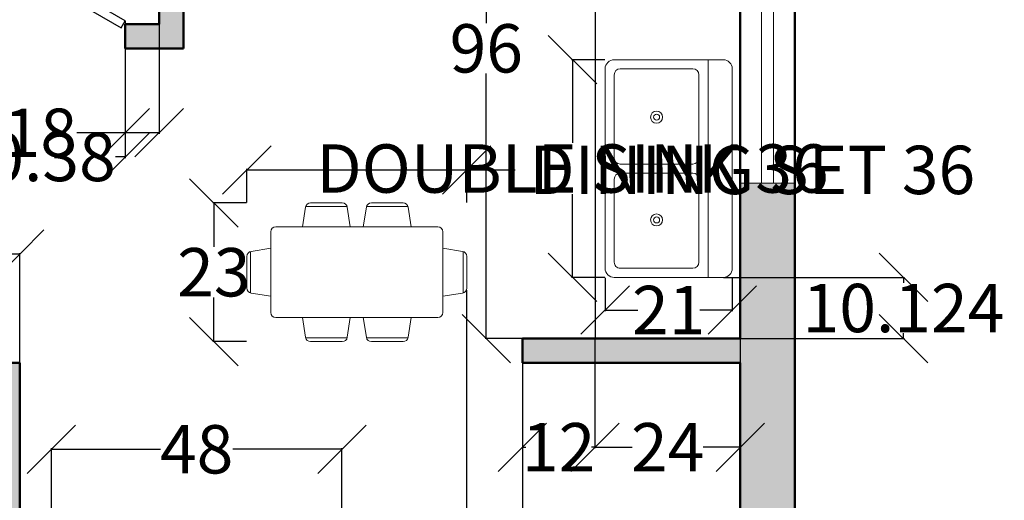
# Model space of a CAD drawing. Units: inches. Extents: x -87 to 308, y -349 to 42.
# Tile 4 of 6: x 119 to 281, y -189 to -110. Entities that reach past the tile are written whole.
import ezdxf

# ---------------------------------------------------------------- set-up
doc = ezdxf.new("R2010")
doc.units = ezdxf.units.IN
doc.header["$MEASUREMENT"] = 0
for name, color, linetype, lineweight in [('A-ANNO-DIMS', 2, 'Continuous', 18), ('A-DOOR', 3, 'Continuous', 25), ('A-FLOR-CASE', 9, 'Continuous', 25), ('A-FLOR-FIXT', 9, 'Continuous', 18), ('A-FURN', 8, 'Continuous', 18), ('A-GLAZ', 4, 'Continuous', 18), ('A-WALL', 7, 'Continuous', 50), ('A-WALL-PATT', 251, 'Continuous', 13)]:
    doc.layers.add(name, color=color, linetype=linetype, lineweight=lineweight)
doc.styles.get("Standard").update_dxf_attribs({"font": 'arial.ttf'})
doc.dimstyles.get("Standard").update_dxf_attribs({"dimtxt": 8, "dimasz": 8, "dimexe": 0.18, "dimexo": 0.0625, "dimgap": 0.09, "dimtad": 0, "dimtih": 1, "dimtoh": 1, "dimdec": 0, "dimzin": 0, "dimdsep": 46, "dimlunit": 4, "dimtxsty": 'Standard', "dimblk": 'OBLIQUE', "dimcen": 0.09, "dimadec": 0, "dimazin": 0, "dimtfac": 1, "dimtdec": 0, "dimtofl": 0, "dimtmove": 0, "dimatfit": 3, "dimldrblk": 'OBLIQUE', "dimfxl": 1, "dimtolj": 1, "dimtzin": 0, "dimarcsym": 0})

# ---------------------------------------------------------------- blocks, each defined once
blk = doc.blocks.new('*U5')
for p, q in [((0, 0), (0, -6)), ((-40, 0), (-40, -6))]:
    blk.add_line(p, q)
blk.add_lwpolyline([(0, 0), (-34.64, 20), (-35.52, 18.48), (-0.88, -1.52)], close=True)
blk.add_arc((0, 0), 40, 150, 180)
blk = doc.blocks.new('Dining Set - 36 x 72 in.')
for p, q in [((-20.29, 27.5), (-7.71, 27.5)), ((3.82, 27.5), (16.4, 27.5)), ((-22.26, 25.81), (-23.48, 18)), ((-22.23, 26), (-5.76, 26)), ((-4.52, 18), (-5.74, 25.81)), ((1.85, 25.81), (0.63, 18)), ((1.88, 26), (18.35, 26)), ((19.6, 18), (18.38, 25.81)), ((-36, 16), (-36, -16)), ((-3.89, 18), (-34, 18)), ((30.11, 18), (-3.89, 18)), ((32.11, -16), (32.11, 16)), ((-44, 8.23), (-44, -8.24)), ((-43.81, 8.26), (-36, 9.48)), ((39.92, 8.26), (32.11, 9.48)), ((40.11, 8.23), (40.11, -8.24)), ((-45.5, 6.29), (-45.5, -6.29)), ((41.61, 6.29), (41.61, -6.29)), ((-36, -9.48), (-43.81, -8.26)), ((32.11, -9.48), (39.92, -8.26)), ((-34, -18), (-3.57, -18)), ((-22.26, -25.81), (-23.48, -18)), ((-4.52, -18), (-5.74, -25.81)), ((-3.89, -18), (30.11, -18)), ((1.85, -25.81), (0.63, -18)), ((19.6, -18), (18.38, -25.81)), ((-22.23, -26), (-5.76, -26)), ((1.88, -26), (18.35, -26)), ((-20.29, -27.5), (-7.71, -27.5)), ((3.82, -27.5), (16.4, -27.5))]:
    blk.add_line(p, q)
for centre, start, end in [((-20.29, 25.5), 90, 171.1198), ((-7.71, 25.5), 8.881, 90), ((3.82, 25.5), 90, 171.1198), ((16.4, 25.5), 8.881, 90), ((-34, 16), 90, 180), ((30.11, 16), 0, 90), ((-43.5, 6.29), 98.8806, 180), ((39.61, 6.29), 0, 81.1194), ((-43.5, -6.29), 180, 261.1194), ((39.61, -6.29), 278.8806, 0), ((-34, -16), 180, 270), ((30.11, -16), 270, 0), ((-20.29, -25.5), 188.8802, 270), ((-7.71, -25.5), 270, 351.1191), ((3.82, -25.5), 188.8802, 270), ((16.4, -25.5), 270, 351.1191)]:
    blk.add_arc(centre, 2, start, end)
blk = doc.blocks.new('Sink-double - 36 in top')
for p, q in [((-18, -4), (18, -4)), ((-0.75, -18.5), (-0.75, -6.5)), ((0.75, -6.5), (0.75, -18.5))]:
    blk.add_line(p, q)
for points in [[(-16.5, 0), (16.5, 0)], [(-18, -19.5), (-18, -1.5)], [(18, -1.5), (18, -19.5)], [(-16.5, -18.5), (-16.5, -6.5)], [(-15.5, -5.5), (-1.75, -5.5)], [(1.75, -5.5), (15.5, -5.5)], [(16.5, -6.5), (16.5, -18.5)], [(-1.75, -19.5), (-15.5, -19.5)], [(15.5, -19.5), (1.75, -19.5)], [(16.5, -21), (-16.5, -21)]]:
    blk.add_lwpolyline(points)
for centre, radius in [((-8.5, -12.5), 1), ((-8.5, -12.5), 0.5), ((8.5, -12.5), 1), ((8.5, -12.5), 0.5)]:
    blk.add_circle(centre, radius)
for centre, radius, start, end in [((-16.5, -1.5), 1.5, 90, 180), ((16.5, -1.5), 1.5, 0, 90), ((-15.5, -6.5), 1, 90, 180), ((-1.75, -6.5), 1, 0, 90), ((1.75, -6.5), 1, 90, 180), ((15.5, -6.5), 1, 0, 90), ((-16.5, -19.5), 1.5, 180, 270), ((-15.5, -18.5), 1, 180, 270), ((-1.75, -18.5), 1, 270, 0), ((1.75, -18.5), 1, 180, 270), ((15.5, -18.5), 1, 270, 0), ((16.5, -19.5), 1.5, 270, 0)]:
    blk.add_arc(centre, radius, start, end)
blk = doc.blocks.new('WIN-48IN')
for p, q in [((0, 5.5), (48, 5.5)), ((0, 3.5), (48, 3.5))]:
    blk.add_line(p, q)
for points in [[(0, 0), (0, 9)], [(48, 9), (48, 0)]]:
    blk.add_lwpolyline(points)
blk = doc.blocks.new('_Oblique')
at = {"color": 0, "linetype": 'ByBlock', "lineweight": -2}
blk.add_line((-0.5, -0.5), (0.5, 0.5), dxfattribs=at)
blk = doc.blocks.new('*D39')
at = {"layer": 'A-ANNO-DIMS', "color": 0, "lineweight": -2, "transparency": 16777216}
for p, q in [((156.24, -140.15), (156.24, -134.59)), ((156.24, -134.77), (192.58, -134.77)), ((192.58, -140.15), (192.58, -134.59)), ((192.58, -134.77), (200.58, -134.77))]:
    blk.add_line(p, q, dxfattribs=at)
at = {"layer": 'Defpoints', "color": 0, "transparency": 16777216}
for p in [(192.58, -134.77), (156.24, -140.22), (192.58, -140.22)]:
    blk.add_point(p, dxfattribs=at)
at = {"layer": 'A-ANNO-DIMS', "color": 0, "lineweight": -2, "transparency": 16777216, "xscale": 8, "yscale": 8, "zscale": 8, "rotation": 180}
blk.add_blockref('_Oblique', (156.24, -134.77), dxfattribs=at)
at = {"layer": 'A-ANNO-DIMS', "color": 0, "lineweight": -2, "transparency": 16777216, "xscale": 8, "yscale": 8, "zscale": 8}
blk.add_blockref('_Oblique', (192.58, -134.77), dxfattribs=at)
at = {"layer": 'A-ANNO-DIMS', "color": 0, "transparency": 16777216, "insert": (239.73, -134.77), "char_height": 8, "attachment_point": 5}
blk.add_mtext('\\A1;DINING SET 36', dxfattribs=at)
blk = doc.blocks.new('*D40')
at = {"layer": 'A-ANNO-DIMS', "color": 0, "lineweight": -2, "transparency": 16777216}
for p, q in [((156.18, -140.22), (150.61, -140.22)), ((150.79, -140.22), (150.79, -147.51)), ((150.79, -163.16), (150.79, -155.87)), ((156.18, -163.16), (150.61, -163.16))]:
    blk.add_line(p, q, dxfattribs=at)
at = {"layer": 'Defpoints', "color": 0, "transparency": 16777216}
for p in [(150.79, -140.22), (156.24, -140.22), (156.24, -163.16)]:
    blk.add_point(p, dxfattribs=at)
at = {"layer": 'A-ANNO-DIMS', "color": 0, "lineweight": -2, "transparency": 16777216, "xscale": 8, "yscale": 8, "zscale": 8}
for p, rotation in [((150.79, -140.22), 90), ((150.79, -163.16), 270)]:
    blk.add_blockref('_Oblique', p, dxfattribs=dict(at, rotation=rotation))
at = {"layer": 'A-ANNO-DIMS', "color": 0, "transparency": 16777216, "insert": (150.79, -151.69), "char_height": 8, "attachment_point": 5}
blk.add_mtext('\\A1;23', dxfattribs=at)
blk = doc.blocks.new('*D43')
at = {"layer": 'A-ANNO-DIMS', "color": 0, "lineweight": -2, "transparency": 16777216}
for p, q in [((215.38, -116.54), (209.86, -116.54)), ((210.04, -116.54), (210.04, -130.31)), ((210.04, -152.54), (210.04, -138.78)), ((215.38, -152.54), (209.86, -152.54))]:
    blk.add_line(p, q, dxfattribs=at)
at = {"layer": 'Defpoints', "color": 0, "transparency": 16777216}
for p in [(215.44, -116.54), (210.04, -152.54), (215.44, -152.54)]:
    blk.add_point(p, dxfattribs=at)
at = {"layer": 'A-ANNO-DIMS', "color": 0, "lineweight": -2, "transparency": 16777216, "xscale": 8, "yscale": 8, "zscale": 8}
for p, rotation in [((210.04, -116.54), 90), ((210.04, -152.54), 270)]:
    blk.add_blockref('_Oblique', p, dxfattribs=dict(at, rotation=rotation))
at = {"layer": 'A-ANNO-DIMS', "color": 0, "transparency": 16777216, "insert": (210.04, -134.54), "char_height": 8, "attachment_point": 5}
blk.add_mtext('\\A1;DOUBLE SINK 36', dxfattribs=at)
blk = doc.blocks.new('*D44')
at = {"layer": 'A-ANNO-DIMS', "color": 0, "lineweight": -2, "transparency": 16777216}
for p, q in [((215.44, -152.61), (215.44, -158.12)), ((236.44, -152.61), (236.44, -158.12)), ((215.44, -157.94), (220.82, -157.94)), ((236.44, -157.94), (231.06, -157.94))]:
    blk.add_line(p, q, dxfattribs=at)
at = {"layer": 'Defpoints', "color": 0, "transparency": 16777216}
for p in [(215.44, -152.54), (236.44, -152.54), (236.44, -157.94)]:
    blk.add_point(p, dxfattribs=at)
at = {"layer": 'A-ANNO-DIMS', "color": 0, "lineweight": -2, "transparency": 16777216, "xscale": 8, "yscale": 8, "zscale": 8, "rotation": 180}
blk.add_blockref('_Oblique', (215.44, -157.94), dxfattribs=at)
at = {"layer": 'A-ANNO-DIMS', "color": 0, "lineweight": -2, "transparency": 16777216, "xscale": 8, "yscale": 8, "zscale": 8}
blk.add_blockref('_Oblique', (236.44, -157.94), dxfattribs=at)
at = {"layer": 'A-ANNO-DIMS', "color": 0, "transparency": 16777216, "insert": (225.94, -157.94), "char_height": 8, "attachment_point": 5}
blk.add_mtext('\\A1;21', dxfattribs=at)
blk = doc.blocks.new('*D58')
at = {"layer": 'A-ANNO-DIMS', "color": 0, "lineweight": -2, "transparency": 16777216}
for p, q in [((21.76, -110.61), (21.76, -92.52)), ((21.76, -92.7), (73.23, -92.7)), ((141.76, -92.7), (90.3, -92.7)), ((141.76, -110.61), (141.76, -92.52))]:
    blk.add_line(p, q, dxfattribs=at)
at = {"layer": 'Defpoints', "color": 0, "transparency": 16777216}
for p in [(141.76, -92.7), (21.76, -110.67), (141.76, -110.67)]:
    blk.add_point(p, dxfattribs=at)
at = {"layer": 'A-ANNO-DIMS', "color": 0, "lineweight": -2, "transparency": 16777216, "xscale": 8, "yscale": 8, "zscale": 8, "rotation": 180}
blk.add_blockref('_Oblique', (21.76, -92.7), dxfattribs=at)
at = {"layer": 'A-ANNO-DIMS', "color": 0, "lineweight": -2, "transparency": 16777216, "xscale": 8, "yscale": 8, "zscale": 8}
blk.add_blockref('_Oblique', (141.76, -92.7), dxfattribs=at)
at = {"layer": 'A-ANNO-DIMS', "color": 0, "transparency": 16777216, "insert": (81.76, -92.7), "char_height": 8, "attachment_point": 5}
blk.add_mtext('\\A1;120', dxfattribs=at)
blk = doc.blocks.new('*D66')
at = {"layer": 'A-ANNO-DIMS', "color": 0, "lineweight": -2, "transparency": 16777216}
for p, q in [((105.76, -114.73), (105.76, -132.81)), ((136.15, -114.73), (136.15, -132.81)), ((105.76, -132.63), (107.36, -132.63)), ((136.15, -132.63), (134.55, -132.63))]:
    blk.add_line(p, q, dxfattribs=at)
at = {"layer": 'Defpoints', "color": 0, "transparency": 16777216}
for p in [(105.76, -114.67), (136.15, -114.67), (105.76, -132.63)]:
    blk.add_point(p, dxfattribs=at)
at = {"layer": 'A-ANNO-DIMS', "color": 0, "lineweight": -2, "transparency": 16777216, "xscale": 8, "yscale": 8, "zscale": 8, "rotation": 180}
blk.add_blockref('_Oblique', (105.76, -132.63), dxfattribs=at)
at = {"layer": 'A-ANNO-DIMS', "color": 0, "lineweight": -2, "transparency": 16777216, "xscale": 8, "yscale": 8, "zscale": 8}
blk.add_blockref('_Oblique', (136.15, -132.63), dxfattribs=at)
at = {"layer": 'A-ANNO-DIMS', "color": 0, "transparency": 16777216, "insert": (120.95, -132.63), "char_height": 8, "attachment_point": 5}
blk.add_mtext('\\A1;30.38', dxfattribs=at)
blk = doc.blocks.new('*D67')
at = {"layer": 'A-ANNO-DIMS', "color": 0, "lineweight": -2, "transparency": 16777216}
for p, q in [((136.15, -110.73), (136.15, -128.81)), ((141.76, -110.73), (141.76, -128.81)), ((136.15, -128.63), (128.15, -128.63)), ((141.76, -128.63), (136.15, -128.63))]:
    blk.add_line(p, q, dxfattribs=at)
at = {"layer": 'Defpoints', "color": 0, "transparency": 16777216}
for p in [(136.15, -110.67), (141.76, -110.67), (136.15, -128.63)]:
    blk.add_point(p, dxfattribs=at)
at = {"layer": 'A-ANNO-DIMS', "color": 0, "lineweight": -2, "transparency": 16777216, "xscale": 8, "yscale": 8, "zscale": 8, "rotation": 180}
blk.add_blockref('_Oblique', (136.15, -128.63), dxfattribs=at)
at = {"layer": 'A-ANNO-DIMS', "color": 0, "lineweight": -2, "transparency": 16777216, "xscale": 8, "yscale": 8, "zscale": 8}
blk.add_blockref('_Oblique', (141.76, -128.63), dxfattribs=at)
at = {"layer": 'A-ANNO-DIMS', "color": 0, "transparency": 16777216, "insert": (114.55, -128.63), "char_height": 8, "attachment_point": 5}
blk.add_mtext('\\A1;5.618', dxfattribs=at)
blk = doc.blocks.new('*D73')
at = {"layer": 'A-ANNO-DIMS', "color": 0, "lineweight": -2, "transparency": 16777216}
for p, q in [((110.71, -166.61), (110.71, -148.52)), ((110.71, -148.7), (111.99, -148.7)), ((118.71, -148.7), (117.44, -148.7)), ((118.71, -166.61), (118.71, -148.52))]:
    blk.add_line(p, q, dxfattribs=at)
at = {"layer": 'Defpoints', "color": 0, "transparency": 16777216}
for p in [(118.71, -148.7), (110.71, -166.67), (118.71, -166.67)]:
    blk.add_point(p, dxfattribs=at)
at = {"layer": 'A-ANNO-DIMS', "color": 0, "lineweight": -2, "transparency": 16777216, "xscale": 8, "yscale": 8, "zscale": 8, "rotation": 180}
blk.add_blockref('_Oblique', (110.71, -148.7), dxfattribs=at)
at = {"layer": 'A-ANNO-DIMS', "color": 0, "lineweight": -2, "transparency": 16777216, "xscale": 8, "yscale": 8, "zscale": 8}
blk.add_blockref('_Oblique', (118.71, -148.7), dxfattribs=at)
at = {"layer": 'A-ANNO-DIMS', "color": 0, "transparency": 16777216, "insert": (114.71, -148.7), "char_height": 8, "attachment_point": 5}
blk.add_mtext('\\A1;8', dxfattribs=at)
blk = doc.blocks.new('*D74')
at = {"layer": 'A-ANNO-DIMS', "color": 0, "lineweight": -2, "transparency": 16777216}
for p, q in [((213.7, -66.67), (195.62, -66.67)), ((195.8, -66.67), (195.8, -110.49)), ((195.8, -162.67), (195.8, -118.84)), ((213.7, -162.67), (195.62, -162.67))]:
    blk.add_line(p, q, dxfattribs=at)
at = {"layer": 'Defpoints', "color": 0, "transparency": 16777216}
for p in [(195.8, -66.67), (213.76, -66.67), (213.76, -162.67)]:
    blk.add_point(p, dxfattribs=at)
at = {"layer": 'A-ANNO-DIMS', "color": 0, "lineweight": -2, "transparency": 16777216, "xscale": 8, "yscale": 8, "zscale": 8}
for p, rotation in [((195.8, -66.67), 90), ((195.8, -162.67), 270)]:
    blk.add_blockref('_Oblique', p, dxfattribs=dict(at, rotation=rotation))
at = {"layer": 'A-ANNO-DIMS', "color": 0, "transparency": 16777216, "insert": (195.8, -114.67), "char_height": 8, "attachment_point": 5}
blk.add_mtext('\\A1;96', dxfattribs=at)
blk = doc.blocks.new('*D75')
at = {"layer": 'A-ANNO-DIMS', "color": 0, "lineweight": -2, "transparency": 16777216}
for p, q in [((213.76, -162.73), (213.76, -180.81)), ((237.76, -162.73), (237.76, -180.81)), ((213.76, -180.63), (219.89, -180.63)), ((237.76, -180.63), (231.64, -180.63))]:
    blk.add_line(p, q, dxfattribs=at)
at = {"layer": 'Defpoints', "color": 0, "transparency": 16777216}
for p in [(213.76, -162.67), (237.76, -162.67), (213.76, -180.63)]:
    blk.add_point(p, dxfattribs=at)
at = {"layer": 'A-ANNO-DIMS', "color": 0, "lineweight": -2, "transparency": 16777216, "xscale": 8, "yscale": 8, "zscale": 8, "rotation": 180}
blk.add_blockref('_Oblique', (213.76, -180.63), dxfattribs=at)
at = {"layer": 'A-ANNO-DIMS', "color": 0, "lineweight": -2, "transparency": 16777216, "xscale": 8, "yscale": 8, "zscale": 8}
blk.add_blockref('_Oblique', (237.76, -180.63), dxfattribs=at)
at = {"layer": 'A-ANNO-DIMS', "color": 0, "transparency": 16777216, "insert": (225.76, -180.63), "char_height": 8, "attachment_point": 5}
blk.add_mtext('\\A1;24', dxfattribs=at)
blk = doc.blocks.new('*D76')
at = {"layer": 'A-ANNO-DIMS', "color": 0, "lineweight": -2, "transparency": 16777216}
for p, q in [((201.76, -162.73), (201.76, -180.81)), ((213.76, -162.73), (213.76, -180.81)), ((201.76, -180.63), (202.36, -180.63)), ((213.76, -180.63), (213.17, -180.63))]:
    blk.add_line(p, q, dxfattribs=at)
at = {"layer": 'Defpoints', "color": 0, "transparency": 16777216}
for p in [(201.76, -162.67), (213.76, -162.67), (201.76, -180.63)]:
    blk.add_point(p, dxfattribs=at)
at = {"layer": 'A-ANNO-DIMS', "color": 0, "lineweight": -2, "transparency": 16777216, "xscale": 8, "yscale": 8, "zscale": 8, "rotation": 180}
blk.add_blockref('_Oblique', (201.76, -180.63), dxfattribs=at)
at = {"layer": 'A-ANNO-DIMS', "color": 0, "lineweight": -2, "transparency": 16777216, "xscale": 8, "yscale": 8, "zscale": 8}
blk.add_blockref('_Oblique', (213.76, -180.63), dxfattribs=at)
at = {"layer": 'A-ANNO-DIMS', "color": 0, "transparency": 16777216, "insert": (207.76, -180.63), "char_height": 8, "attachment_point": 5}
blk.add_mtext('\\A1;12', dxfattribs=at)
blk = doc.blocks.new('*D77')
at = {"layer": 'A-ANNO-DIMS', "color": 0, "lineweight": -2, "transparency": 16777216}
for p, q in [((123.95, -198.87), (123.95, -180.79)), ((123.95, -180.97), (141.96, -180.97)), ((171.95, -180.97), (153.94, -180.97)), ((171.95, -198.87), (171.95, -180.79))]:
    blk.add_line(p, q, dxfattribs=at)
at = {"layer": 'Defpoints', "color": 0, "transparency": 16777216}
for p in [(171.95, -180.97), (123.95, -198.94), (171.95, -198.94)]:
    blk.add_point(p, dxfattribs=at)
at = {"layer": 'A-ANNO-DIMS', "color": 0, "lineweight": -2, "transparency": 16777216, "xscale": 8, "yscale": 8, "zscale": 8, "rotation": 180}
blk.add_blockref('_Oblique', (123.95, -180.97), dxfattribs=at)
at = {"layer": 'A-ANNO-DIMS', "color": 0, "lineweight": -2, "transparency": 16777216, "xscale": 8, "yscale": 8, "zscale": 8}
blk.add_blockref('_Oblique', (171.95, -180.97), dxfattribs=at)
at = {"layer": 'A-ANNO-DIMS', "color": 0, "transparency": 16777216, "insert": (147.95, -180.97), "char_height": 8, "attachment_point": 5}
blk.add_mtext('\\A1;48', dxfattribs=at)
blk = doc.blocks.new('*D89')
at = {"layer": 'A-ANNO-DIMS', "color": 0, "lineweight": -2, "transparency": 16777216}
for p, q in [((235, -152.54), (264.91, -152.54)), ((264.73, -152.54), (264.73, -153.43)), ((237.83, -162.67), (264.91, -162.67)), ((264.73, -162.67), (264.73, -161.78))]:
    blk.add_line(p, q, dxfattribs=at)
at = {"layer": 'Defpoints', "color": 0, "transparency": 16777216}
for p in [(234.94, -152.54), (237.76, -162.67), (264.73, -162.67)]:
    blk.add_point(p, dxfattribs=at)
at = {"layer": 'A-ANNO-DIMS', "color": 0, "lineweight": -2, "transparency": 16777216, "xscale": 8, "yscale": 8, "zscale": 8}
for p, rotation in [((264.73, -152.54), 90), ((264.73, -162.67), 270)]:
    blk.add_blockref('_Oblique', p, dxfattribs=dict(at, rotation=rotation))
at = {"layer": 'A-ANNO-DIMS', "color": 0, "transparency": 16777216, "insert": (264.73, -157.61), "char_height": 8, "attachment_point": 5}
blk.add_mtext('\\A1;10.124', dxfattribs=at)
blk = doc.blocks.new('*D94')
at = {"layer": 'A-ANNO-DIMS', "color": 0, "lineweight": -2, "transparency": 16777216}
for p, q in [((192.53, -154.67), (192.53, -341.81)), ((201.76, -162.73), (201.76, -341.81)), ((192.53, -341.63), (201.76, -341.63)), ((201.76, -341.63), (209.76, -341.63))]:
    blk.add_line(p, q, dxfattribs=at)
at = {"layer": 'Defpoints', "color": 0, "transparency": 16777216}
for p in [(192.53, -154.61), (201.76, -162.67), (201.76, -341.63)]:
    blk.add_point(p, dxfattribs=at)
at = {"layer": 'A-ANNO-DIMS', "color": 0, "lineweight": -2, "transparency": 16777216, "xscale": 8, "yscale": 8, "zscale": 8, "rotation": 180}
blk.add_blockref('_Oblique', (192.53, -341.63), dxfattribs=at)
at = {"layer": 'A-ANNO-DIMS', "color": 0, "lineweight": -2, "transparency": 16777216, "xscale": 8, "yscale": 8, "zscale": 8}
blk.add_blockref('_Oblique', (201.76, -341.63), dxfattribs=at)
at = {"layer": 'A-ANNO-DIMS', "color": 0, "transparency": 16777216, "insert": (223.34, -341.63), "char_height": 8, "attachment_point": 5}
blk.add_mtext('\\A1;9.234', dxfattribs=at)

msp = doc.modelspace()

# ---------------------------------------------------------------- hatches: boundary and pattern name
at = {"layer": 'A-WALL-PATT'}
h = msp.add_hatch(color=256, dxfattribs=at)
h.dxf.hatch_style = 1
h.paths.add_polyline_path([(184.748, 18.332), (84.6671, 18.332), (84.6671, 9.332), (141.7637, 9.332), (141.7637, -110.668), (136.146, -110.668), (136.146, -114.668), (145.7637, -114.668), (145.7637, -66.668), (151.7637, -66.668), (151.7637, -62.668), (145.7637, -62.668), (145.7637, 9.332), (184.748, 9.332)])
h = msp.add_hatch(color=256, dxfattribs=at)
h.dxf.hatch_style = 1
h.paths.add_polyline_path([(246.7637, -136.9351), (237.7637, -136.9351), (237.7637, -162.668), (237.7637, -166.668), (237.7637, -314.668), (237.6195, -323.668), (246.7637, -323.668)])
h = msp.add_hatch(color=256, dxfattribs=at)
h.dxf.hatch_style = 1
h.paths.add_polyline_path([(237.7637, -162.668), (213.7637, -162.668), (201.7637, -162.668), (201.7637, -166.668), (213.7637, -166.668), (237.7637, -166.668)])
h = msp.add_hatch(color=256, dxfattribs=at)
h.dxf.hatch_style = 1
h.paths.add_polyline_path([(118.7127, -170.668), (118.7127, -166.668), (114.7127, -166.668), (110.7127, -166.668), (110.7127, -170.668), (114.7127, -170.668), (114.7127, -314.668), (88.2177, -314.668), (88.2177, -323.668), (142.7127, -323.668), (142.7127, -319.1107), (142.7127, -314.668), (118.7127, -314.668)])

# ---------------------------------------------------------------- linework, layer by layer
at = {"layer": 'A-FLOR-CASE'}
msp.add_line((213.7637, -66.668), (213.7637, -162.668), dxfattribs=at)
at = {"layer": 'A-WALL'}
for p, q in [((141.7637, -110.668), (141.7637, 9.332)), ((237.7637, 9.332), (237.7637, -162.668)), ((145.7637, -114.668), (145.7637, -66.668)), ((136.146, -110.668), (141.7637, -110.668)), ((136.146, -110.668), (136.146, -114.668)), ((136.146, -114.668), (145.7637, -114.668)), ((213.7637, -162.668), (201.7637, -162.668)), ((201.7637, -162.668), (201.7637, -166.668)), ((213.7637, -162.668), (237.7637, -162.668)), ((114.7127, -166.668), (118.7127, -166.668)), ((118.7127, -166.668), (118.7127, -170.668)), ((201.7637, -166.668), (213.7637, -166.668)), ((213.7637, -166.668), (237.7637, -166.668)), ((237.7637, -166.668), (237.7637, -314.668)), ((118.7127, -170.668), (118.7127, -314.668))]:
    msp.add_line(p, q, dxfattribs=at)
msp.add_lwpolyline([(142.7127, -323.668), (12.7637, -323.668), (12.7637, 18.332), (246.7637, 18.332), (246.7637, -323.668), (172.7127, -323.668)], dxfattribs=at)

# ---------------------------------------------------------------- block references
at = {"layer": 'A-DOOR', "xscale": 0.7595575434647344, "yscale": 0.7595575434647344, "zscale": 0.7595575434647344}
msp.add_blockref('*U5', (136.146, -110.1107), dxfattribs=at)
at = {"layer": 'A-FLOR-FIXT', "rotation": 270}
msp.add_blockref('Sink-double - 36 in top', (236.44, -134.5443), dxfattribs=at)
at = {"layer": 'A-FURN', "xscale": 0.4171476692869815, "yscale": 0.4171476692869815, "zscale": 0.4171476692869815}
msp.add_blockref('Dining Set - 36 x 72 in.', (175.2243, -151.6889), dxfattribs=at)
at = {"layer": 'A-GLAZ', "rotation": 270.0000000000002}
msp.add_blockref('WIN-48IN', (237.7637, -88.935), dxfattribs=at)

# ---------------------------------------------------------------- dimensions: what is measured, and where the dimension line sits
at = {"layer": 'A-ANNO-DIMS'}
for base, p1, p2, angle, override, picture, middle in [((195.7992, -66.668), (213.7637, -162.668), (213.7637, -66.668), 90, {"dimdec": 0, "dimlfac": 1, "dimrnd": 0, "dimzin": 0, "dimdsep": 46, "dimlunit": 2}, '*D74', (195.7992, -114.668)), ((136.146, -128.6325), (141.7637, -110.668), (136.146, -110.668), 180, {"dimdec": 3, "dimlfac": 1, "dimrnd": 0, "dimzin": 0, "dimdsep": 46, "dimlunit": 2}, '*D67', (114.5498, -128.6325)), ((105.7637, -132.6325), (136.146, -114.668), (105.7637, -114.668), 180, {"dimdec": 2, "dimlfac": 1, "dimrnd": 0, "dimzin": 0, "dimdsep": 46, "dimlunit": 2}, '*D66', (120.9548, -132.6325)), ((150.7934, -140.2174), (156.2441, -163.1605), (156.2441, -140.2174), 90, {"dimdec": 0, "dimlfac": 1, "dimrnd": 0, "dimzin": 0, "dimdsep": 46, "dimlunit": 2}, '*D40', (150.7934, -151.6889)), ((118.7127, -148.7035), (110.7127, -166.668), (118.7127, -166.668), 0, {"dimdec": 0, "dimlfac": 1, "dimrnd": 0, "dimzin": 0, "dimdsep": 46, "dimlunit": 2}, '*D73', (114.7127, -148.7035)), ((264.7282, -162.668), (234.94, -152.5443), (237.7637, -162.668), 90, {"dimdec": 3, "dimlfac": 1, "dimrnd": 0, "dimzin": 0, "dimdsep": 46, "dimlunit": 2}, '*D89', (264.7282, -157.6062)), ((201.7637, -180.6325), (213.7637, -162.668), (201.7637, -162.668), 180, {"dimdec": 0, "dimlfac": 1, "dimrnd": 0, "dimzin": 0, "dimdsep": 46, "dimlunit": 2}, '*D76', (207.7637, -180.6325)), ((213.7637, -180.6325), (237.7637, -162.668), (213.7637, -162.668), 180, {"dimdec": 0, "dimlfac": 1, "dimrnd": 0, "dimzin": 0, "dimdsep": 46, "dimlunit": 2}, '*D75', (225.7637, -180.6325))]:
    dim = msp.add_linear_dim(base=base, p1=p1, p2=p2, angle=angle, dimstyle='Standard', override=override, dxfattribs=at)
    dim.commit()
    dim.dimension.update_dxf_attribs({"geometry": picture, "text_midpoint": middle})
for base, p1, p2, override, picture, middle in [((141.7637, -92.7035), (21.7637, -110.668), (141.7637, -110.668), {"dimdec": 0, "dimlfac": 1, "dimrnd": 0, "dimzin": 0, "dimdsep": 46, "dimlunit": 2}, '*D58', (81.7637, -92.7035)), ((236.44, -157.9443), (215.44, -152.5443), (236.44, -152.5443), {"dimdec": 0, "dimlfac": 1, "dimrnd": 0, "dimzin": 0, "dimdsep": 46, "dimlunit": 2}, '*D44', (225.94, -157.9443)), ((201.7637, -341.6325), (192.5294, -154.6053), (201.7637, -162.668), {"dimdec": 3, "dimlfac": 1, "dimrnd": 0, "dimzin": 0, "dimdsep": 46, "dimlunit": 2}, '*D94', (223.3352, -341.6325)), ((171.9465, -180.9706), (123.9465, -198.9351), (171.9465, -198.9351), {"dimdec": 0, "dimlfac": 1, "dimrnd": 0, "dimzin": 0, "dimdsep": 46, "dimlunit": 2}, '*D77', (147.9465, -180.9706))]:
    dim = msp.add_linear_dim(base=base, p1=p1, p2=p2, dimstyle='Standard', override=override, dxfattribs=at)
    dim.commit()
    dim.dimension.update_dxf_attribs({"geometry": picture, "text_midpoint": middle})
dim = msp.add_linear_dim(base=(210.04, -152.5443), p1=(215.44, -116.5443), p2=(215.44, -152.5443), angle=270, text='DOUBLE SINK <>', dimstyle='Standard', override={"dimdec": 0, "dimlfac": 1, "dimrnd": 0, "dimzin": 0, "dimdsep": 46, "dimlunit": 2}, dxfattribs=at)
dim.commit()
dim.dimension.update_dxf_attribs({"geometry": '*D43', "text_midpoint": (210.04, -134.5443)})
dim = msp.add_linear_dim(base=(192.5825, -134.7666), p1=(156.2441, -140.2174), p2=(192.5825, -140.2174), text='DINING SET <>', dimstyle='Standard', override={"dimdec": 0, "dimlfac": 1, "dimrnd": 0, "dimzin": 0, "dimdsep": 46, "dimlunit": 2}, dxfattribs=at)
dim.commit()
dim.dimension.update_dxf_attribs({"geometry": '*D39', "text_midpoint": (239.7312, -134.7666)})

doc.saveas('drawing.dxf')
